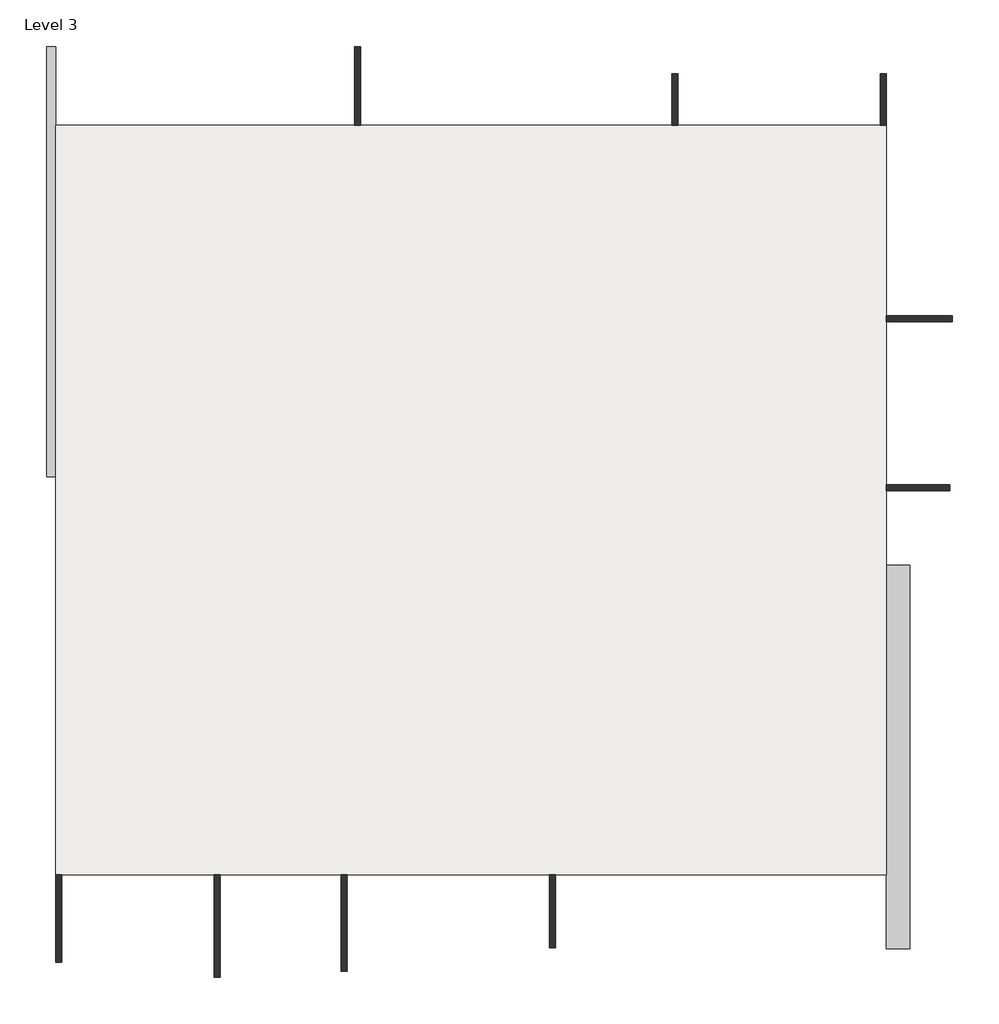
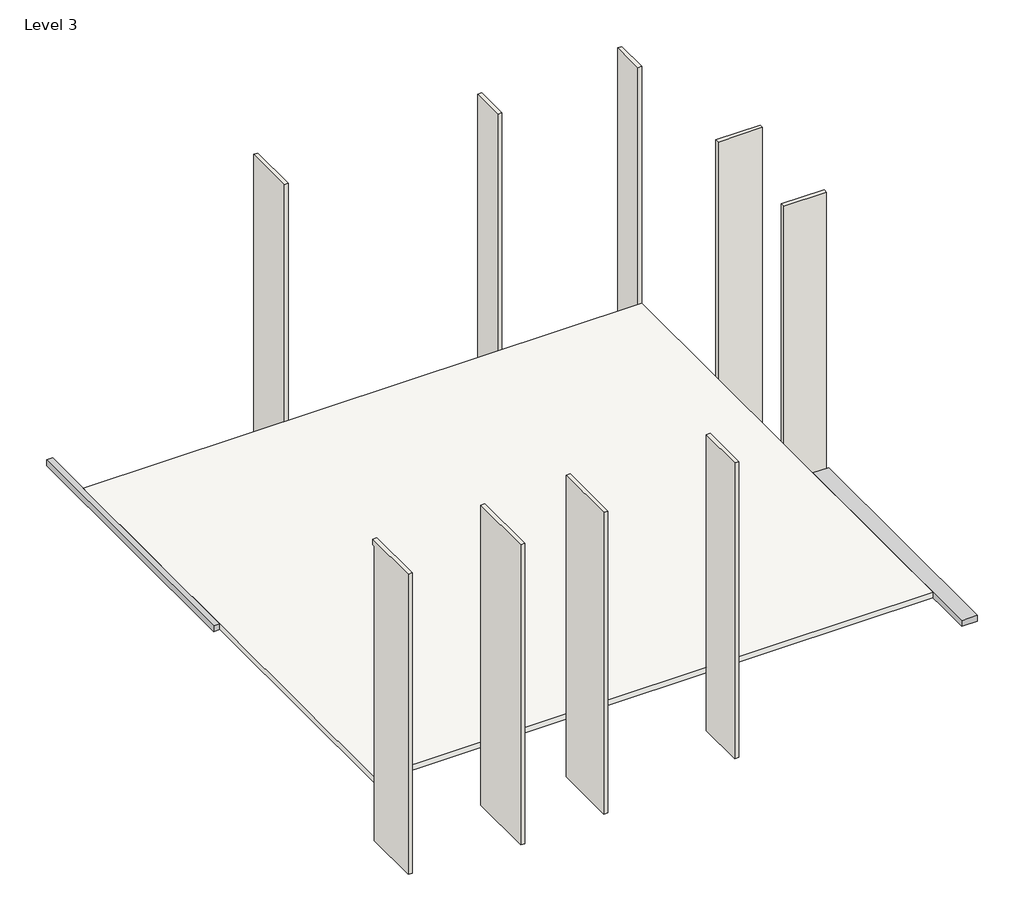
# One storey: 9 walls, 2 proxies, 1 slab.
"""IFC4 building model written with IfcOpenShell, lengths in millimetres."""

from ifc_helpers import new_model, si_unit, frame, origin, place, context, project, spatial, polyline, outline, extrude, transform, mapped, element, save
from components import generic_models_12_generic_models_12_d8093b74, generic_models_4_generic_models_4_f29f5d5a

model = new_model("IFC4")

# Units and contexts
model_context = context("Model", 3, world=origin())
ifc_project = project(units=[si_unit("LENGTHUNIT", "METRE", prefix="MILLI")], contexts=[model_context])

# Site, building, storey
site = spatial("IfcSite", under=ifc_project)
building = spatial("IfcBuilding", under=site)
storey = spatial("IfcBuildingStorey", under=building, Name="Level 3", Elevation=6096.0)

# Proxies
placement = place(None, origin())
generic_models_12_generic_models_12_shape = generic_models_12_generic_models_12_d8093b74(model_context)
element("IfcBuildingElementProxy", 1, Name="Generic Models 12 : Generic Models 12", ObjectType="Generic Models 12 : Generic Models 12", at=placement, inside=storey, context=model_context, shape_type="MappedRepresentation", body=[
    mapped(generic_models_12_generic_models_12_shape, transform((0.0, 0.0, 0.0), x_axis=(1.0, 0.0, 0.0), y_axis=(0.0, 1.0, 0.0), z_axis=(0.0, 0.0, 1.0))),
])
generic_models_4_generic_models_4_shape = generic_models_4_generic_models_4_f29f5d5a(model_context)
element("IfcBuildingElementProxy", 2, Name="Generic Models 4 : Generic Models 4", ObjectType="Generic Models 4 : Generic Models 4", at=placement, inside=storey, context=model_context, shape_type="MappedRepresentation", body=[
    mapped(generic_models_4_generic_models_4_shape, transform((0.0, 0.0, 0.0), x_axis=(1.0, 0.0, 0.0), y_axis=(0.0, 1.0, 0.0), z_axis=(0.0, 0.0, 1.0))),
])

# Slab
element("IfcSlab", 3, ObjectType="Generic - 12\"", at=placement, inside=storey, context=model_context, shape_type="SweptSolid", body=[
    extrude(outline(polyline([(14106.5361222, 14768.6237525), (14106.5361222, -10428.1762475), (-13833.4638778, -10428.1762475), (-13833.4638778, 14768.6237525), (14106.5361222, 14768.6237525)])), frame((0.0, 0.0, 6096.0), z_axis=(0.0, 0.0, 1.0), x_axis=(1.0, 0.0, 0.0)), (0.0, 0.0, 1.0), 304.8),
])

# Walls
element("IfcWall", 4, ObjectType="Generic - 8\"", at=placement, inside=storey, context=model_context, shape_type="SweptSolid", body=[
    extrude(outline(polyline([(-10428.1762475, 3048.0), (-13374.5762475, 3048.0), (-13374.5762475, 18918.7849443), (-10326.5762475, 18918.7849443), (-10326.5762475, 18613.9849443), (-10428.1762475, 18613.9849443), (-10428.1762475, 3048.0)])), frame((-13833.4638778, 0.0, 0.0), z_axis=(1.0, 0.0, 0.0), x_axis=(0.0, 1.0, 0.0)), (0.0, 0.0, 1.0), 203.2),
])
element("IfcWall", 5, ObjectType="Generic - 8\"", at=placement, inside=storey, context=model_context, shape_type="SweptSolid", body=[
    extrude(outline(polyline([(-8499.4638778, -13882.5762475), (-8499.4638778, -10428.1762475), (-8296.2638778, -10428.1762475), (-8296.2638778, -13882.5762475), (-8499.4638778, -13882.5762475)])), frame((0.0, 0.0, 3048.0), z_axis=(0.0, 0.0, 1.0), x_axis=(1.0, 0.0, 0.0)), (0.0, 0.0, 1.0), 15870.7849443),
])
element("IfcWall", 6, ObjectType="Generic - 8\"", at=placement, inside=storey, context=model_context, shape_type="SweptSolid", body=[
    extrude(outline(polyline([(-4232.2638778, -13679.3762475), (-4232.2638778, -10428.1762475), (-4029.0638778, -10428.1762475), (-4029.0638778, -13679.3762475), (-4232.2638778, -13679.3762475)])), frame((0.0, 0.0, 3048.0), z_axis=(0.0, 0.0, 1.0), x_axis=(1.0, 0.0, 0.0)), (0.0, 0.0, 1.0), 15958.5942777),
])
element("IfcWall", 7, ObjectType="Generic - 8\"", at=placement, inside=storey, context=model_context, shape_type="SweptSolid", body=[
    extrude(outline(polyline([(2778.1361222, -12886.3749501), (2778.1361222, -10428.1762475), (2981.3361222, -10428.1762475), (2981.3361222, -12886.3749501), (2778.1361222, -12886.3749501)])), frame((0.0, 0.0, 3048.0), z_axis=(0.0, 0.0, 1.0), x_axis=(1.0, 0.0, 0.0)), (0.0, 0.0, 1.0), 15643.5031982),
])
element("IfcWall", 8, ObjectType="Generic - 8\"", at=placement, inside=storey, context=model_context, shape_type="SweptSolid", body=[
    extrude(outline(polyline([(16240.1361222, 2475.0237525), (14106.5361222, 2475.0237525), (14106.5361222, 2678.2237525), (16240.1361222, 2678.2237525), (16240.1361222, 2475.0237525)])), frame((0.0, 0.0, 3048.0), z_axis=(0.0, 0.0, 1.0), x_axis=(1.0, 0.0, 0.0)), (0.0, 0.0, 1.0), 15926.7979205),
])
element("IfcWall", 9, ObjectType="Generic - 8\"", at=placement, inside=storey, context=model_context, shape_type="SweptSolid", body=[
    extrude(outline(polyline([(16321.4289933, 8164.6237525), (14106.5361222, 8164.6237525), (14106.5361222, 8367.8237525), (16321.4289933, 8367.8237525), (16321.4289933, 8164.6237525)])), frame((0.0, 0.0, 3048.0), z_axis=(0.0, 0.0, 1.0), x_axis=(1.0, 0.0, 0.0)), (0.0, 0.0, 1.0), 15870.7849443),
])
element("IfcWall", 10, ObjectType="Generic - 8\"", at=placement, inside=storey, context=model_context, shape_type="SweptSolid", body=[
    extrude(outline(polyline([(14106.5361222, 16495.8237525), (14106.5361222, 14768.6237525), (13903.3361222, 14768.6237525), (13903.3361222, 16495.8237525), (14106.5361222, 16495.8237525)])), frame((0.0, 0.0, 3048.0), z_axis=(0.0, 0.0, 1.0), x_axis=(1.0, 0.0, 0.0)), (0.0, 0.0, 1.0), 15870.7849443),
])
element("IfcWall", 11, ObjectType="Generic - 8\"", at=placement, inside=storey, context=model_context, shape_type="SweptSolid", body=[
    extrude(outline(polyline([(7096.1361222, 16495.8237525), (7096.1361222, 14768.6237525), (6892.9361222, 14768.6237525), (6892.9361222, 16495.8237525), (7096.1361222, 16495.8237525)])), frame((0.0, 0.0, 3048.0), z_axis=(0.0, 0.0, 1.0), x_axis=(1.0, 0.0, 0.0)), (0.0, 0.0, 1.0), 15870.7849443),
])
element("IfcWall", 12, ObjectType="Generic - 8\"", at=placement, inside=storey, context=model_context, shape_type="SweptSolid", body=[
    extrude(outline(polyline([(-3571.8638778, 17410.2237525), (-3571.8638778, 14768.6237525), (-3775.0638778, 14768.6237525), (-3775.0638778, 17410.2237525), (-3571.8638778, 17410.2237525)])), frame((0.0, 0.0, 3048.0), z_axis=(0.0, 0.0, 1.0), x_axis=(1.0, 0.0, 0.0)), (0.0, 0.0, 1.0), 15870.7849443),
])

save(model, "model.ifc")

# Revit data of these elements
# Type "Generic - 12\""
#   Assembly Code = "B1010"
#   Function = 0
#   Layers, outside or top first: 1' - 0" no material (function 1)
# Type "Generic - 8\""
#   Assembly Code = "B2010"
#   Layers, outside or top first: 0' - 8" no material (function 1)
# Element 1 (IfcBuildingElementProxy, "Generic Models 12 : Generic Models 12")
#   Phase Created = New Construction
# Element 2 (IfcBuildingElementProxy, "Generic Models 4 : Generic Models 4")
#   Phase Created = New Construction
# Element 3 (IfcSlab, "Generic - 12\"")
#   Height Offset From Level = 1' - 0"
#   Phase Created = New Construction
#   Materials on its faces: "Default Floor"
# Elements 4, 5, 9, 10, 11, 12 (IfcWall, "Generic - 8\"")
#   built-in parameter 1001111 = -10' - 0"
#   Top Offset = 0' - 0"
#   Base Offset = -10' - 0"
#   Unconnected Height = 52' - 0.83405"
#   wall height = 52' - 0.83405"
#   Phase Created = New Construction
#   Base Constraint = Level 3
#   Materials on its faces: "Default Wall"
# Element 6 (IfcWall, "Generic - 8\"")
#   built-in parameter 1001111 = -10' - 0"
#   Top Offset = 0' - 0"
#   Base Offset = -10' - 0"
#   Unconnected Height = 52' - 4.29111"
#   wall height = 52' - 4.29111"
#   Phase Created = New Construction
#   Base Constraint = Level 3
#   Materials on its faces: "Default Wall"
# Element 7 (IfcWall, "Generic - 8\"")
#   built-in parameter 1001111 = -10' - 0"
#   Top Offset = 0' - 0"
#   Base Offset = -10' - 0"
#   Unconnected Height = 51' - 3.88595"
#   wall height = 51' - 3.88595"
#   Phase Created = New Construction
#   Base Constraint = Level 3
#   Materials on its faces: "Default Wall"
# Element 8 (IfcWall, "Generic - 8\"")
#   built-in parameter 1001111 = -10' - 0"
#   Top Offset = 0' - 0"
#   Base Offset = -10' - 0"
#   Unconnected Height = 52' - 3.03929"
#   wall height = 52' - 3.03929"
#   Phase Created = New Construction
#   Base Constraint = Level 3
#   Materials on its faces: "Default Wall"
# Materials
#   "Default Floor": colour RGB 128 128 128, transparency 0
#   "Default Wall": colour RGB 128 128 128, transparency 0
